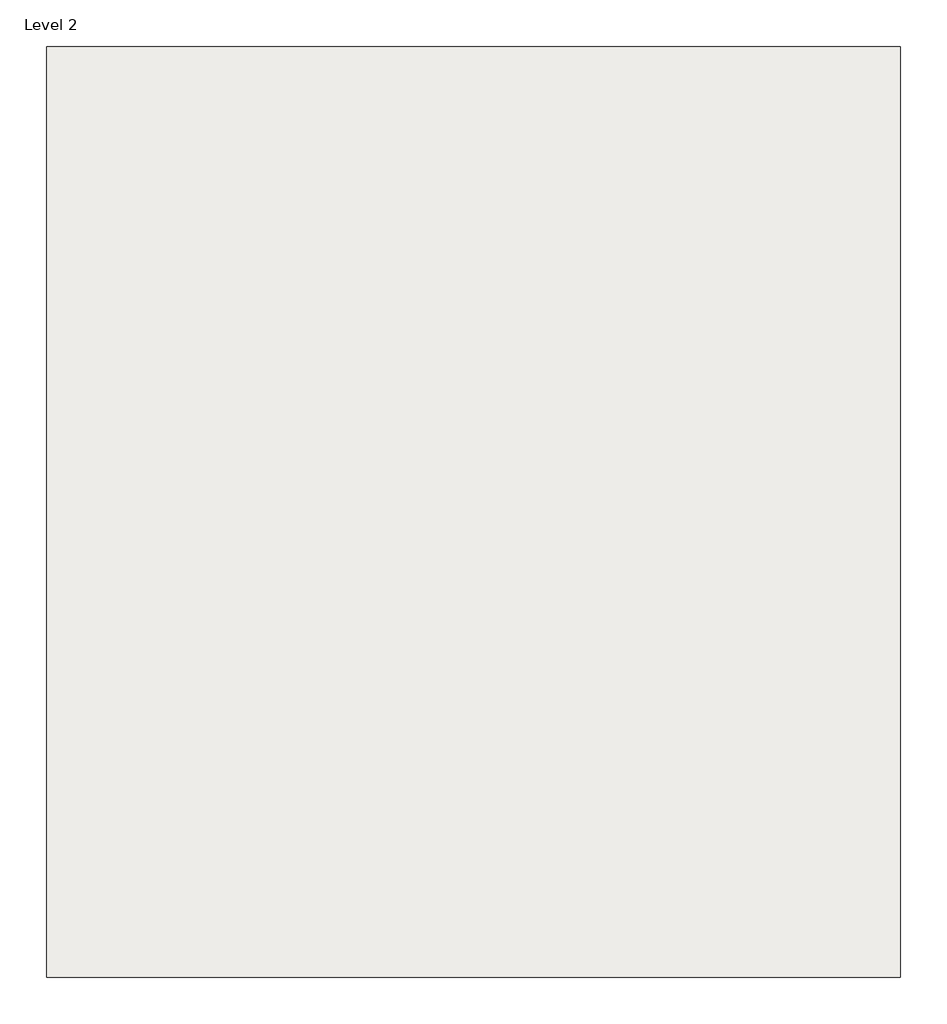
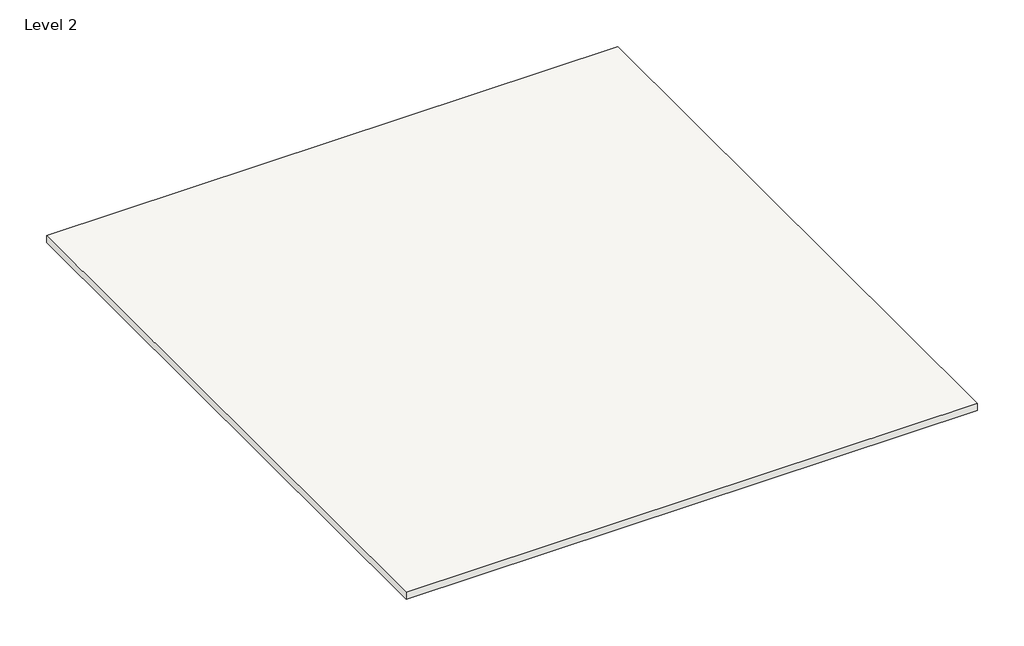
# One storey, incomplete: 1 roof.
"""IFC4 building model written with IfcOpenShell, lengths in millimetres."""

from ifc_helpers import new_model, si_unit, frame, origin, place, context, project, spatial, polyline, outline, extrude, element, save

model = new_model("IFC4")

# Units and contexts
model_context = context("Model", 3, world=origin())
ifc_project = project(units=[si_unit("LENGTHUNIT", "METRE", prefix="MILLI")], contexts=[model_context])

# Site, building, storey
site = spatial("IfcSite", under=ifc_project)
building = spatial("IfcBuilding", under=site)
storey = spatial("IfcBuildingStorey", under=building, Name="Level 2", Elevation=3048.0)

# Roof
placement = place(None, origin())
element("IfcRoof", 1, ObjectType="Generic - 12\"", at=placement, inside=storey, context=model_context, shape_type="SweptSolid", body=[
    extrude(outline(polyline([(-7252.5317864, 7748.8034997), (4771.8282136, 7748.8034997), (4771.8282136, -5357.5965003), (-7252.5317864, -5357.5965003), (-7252.5317864, 7748.8034997)])), frame((0.0, 0.0, 3048.0), z_axis=(0.0, 0.0, 1.0), x_axis=(1.0, 0.0, 0.0)), (0.0, 0.0, 1.0), 152.4),
])

save(model, "model.ifc")

# Revit data of these elements
# Type "Generic - 12\""
#   Assembly Code = "B1020"
#   Layers, outside or top first: 0' - 6" no material (function 1)
# Element 1 (IfcRoof, "Generic - 12\"")
#   built-in parameter 1001705 = 10.5 (stored number, unit not read)
#   built-in parameter 1001710 = 33615
#   Phase Created = New Construction
#   Materials on its faces: "Default Roof"
# Materials
#   "Default Roof": colour RGB 88 101 114, transparency 0, Cost = 0
